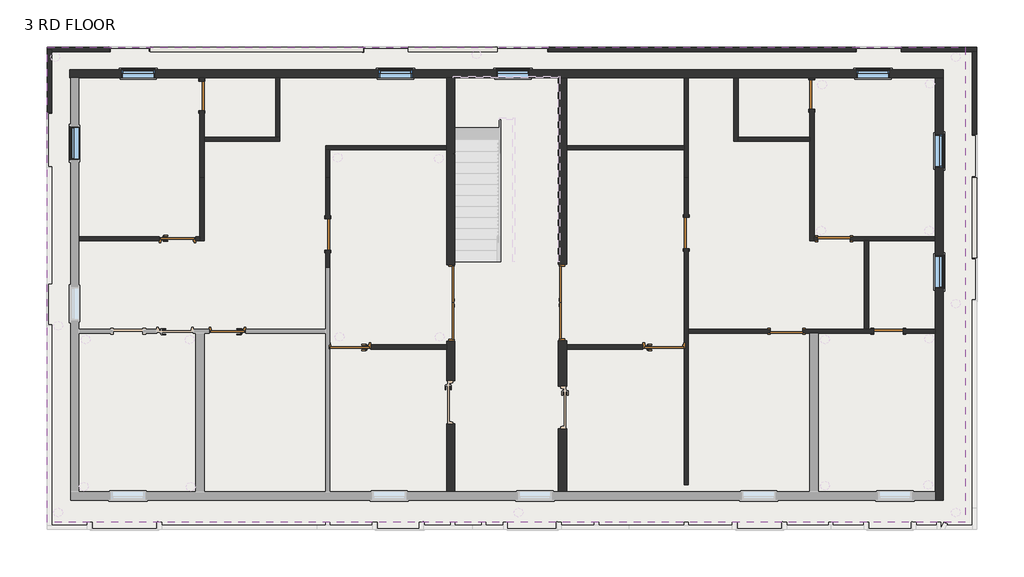
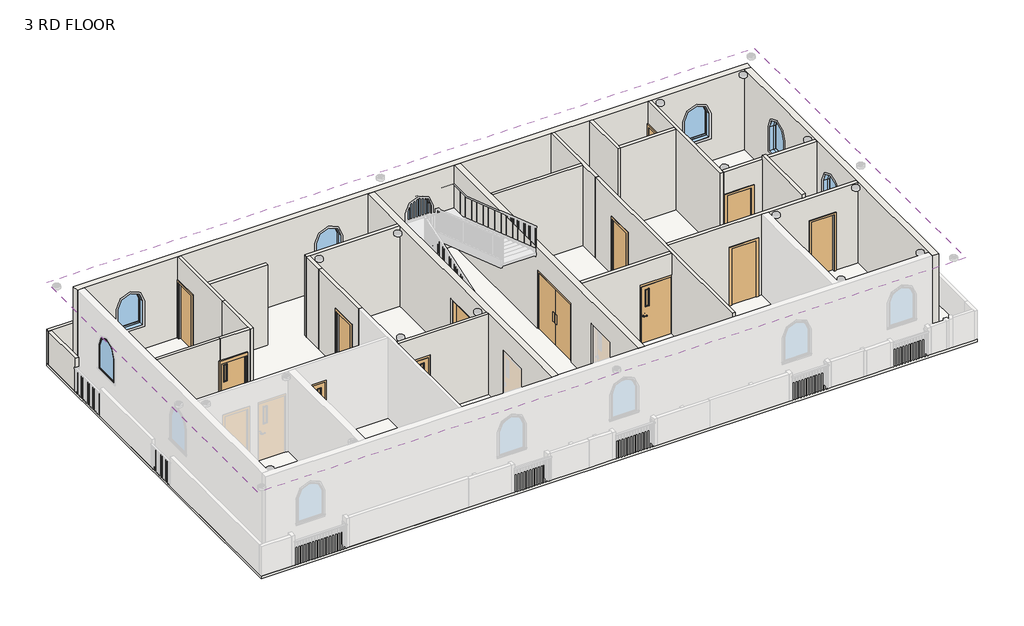
# One storey, part 2 of 7: 33 walls, 13 doors, 7 windows, 1 covering, 1 slab.
# Revit data of these elements (continued)
# Elements 4, 5 (IfcDoor, "Door-Passage-Single-Vision_Lite : 3'6\"X7' 2")
#   Swing Angle = 90.00°
#   Rough Width = 3' - 10"
#   Rough Height = 7' - 4"
#   Masonry Inset = 0' - 1"
#   MFOpeningWidth = 0' - 4"
#   MFOpeningHeight = 0' - 4"
#   Inset Calculate = 0' - 4"
#   Masonry Frame = yes
#   Dry Wall Frame = no
#   Phase Created = New Construction
#   Materials on its faces: "Metal - Paint Finish - Grey", "Aluminum", "Wood - Birch", "Glass"
# Elements 6, 7 (IfcDoor, "Door-Passage-Single-Vision_Lite : 3'X7'")
#   Swing Angle = 90.00°
#   Rough Width = 3' - 4"
#   Rough Height = 7' - 4"
#   Masonry Inset = 0' - 1"
#   MFOpeningWidth = 0' - 4"
#   MFOpeningHeight = 0' - 4"
#   Inset Calculate = 0' - 4"
#   Masonry Frame = yes
#   Dry Wall Frame = no
#   Phase Created = New Construction
#   Materials on its faces: "Metal - Paint Finish - Grey", "Aluminum", "Wood - Birch", "Glass"
# Elements 8, 9 (IfcDoor, "Single-Flush : 2'10\" x 7'")
#   Phase Created = New Construction
#   Materials on its faces: "Door - Frame", "Door - Panel"
# Elements 10, 11 (IfcDoor, "Single-Flush : 2'11\"x 7'")
#   Phase Created = New Construction
#   Materials on its faces: "Door - Frame", "Door - Panel"
# Elements 12, 13, 14 (IfcDoor, "Single-Flush : 2'8\"x 7'")
#   Phase Created = New Construction
#   Materials on its faces: "Door - Frame", "Door - Panel"
# Element 15 (IfcSlab, "LW Concrete on Metal Deck")
#   Height Offset From Level = 0' - 0"
#   Phase Created = New Construction
#   Materials on its faces: "Metal Deck", "Concrete, Lightweight"
# Elements 16, 17, 18, 19, 20, 21, 22, 23, 24, 25, 26, 27, 28, 29, 30, 32, 33, 34 (IfcWall, "Generic - 4.5\"")
#   Top Offset = -0' - 6"
#   Base Offset = 0' - 0"
#   wall height = 10' - 0"
#   Phase Created = New Construction
#   Base Constraint = 3 RD FLOOR
#   Top Constraint = 4 TH FLOOR
#   Materials on its faces: "Default Wall"
# Elements 31, 41 (IfcWall, "Generic - 4.5\"")
#   Top Offset = -6' - 0"
#   Base Offset = 0' - 0"
#   wall height = 4' - 6"
#   Phase Created = New Construction
#   Base Constraint = 3 RD FLOOR
#   Top Constraint = 4 TH FLOOR
#   Materials on its faces: "Default Wall"
# Element 35 (IfcWall, "Generic - 4.5\"")
#   Top Offset = -6' - 4.43284"
#   Base Offset = 0' - 0"
#   wall height = 4' - 1.56716"
#   Phase Created = New Construction
#   Base Constraint = 3 RD FLOOR
#   Top Constraint = 4 TH FLOOR
#   Materials on its faces: "Default Wall"
# Element 36 (IfcWall, "Generic - 4.5\"")
#   Top Offset = -6' - 3.86561"
#   Base Offset = 0' - 0"
#   wall height = 4' - 2.13439"
#   Phase Created = New Construction
#   Base Constraint = 3 RD FLOOR
#   Top Constraint = 4 TH FLOOR
#   Materials on its faces: "Default Wall"
# Element 37 (IfcWall, "Generic - 4.5\"")
#   Top Offset = -6' - 11.32684"
#   Base Offset = 0' - 0"
#   wall height = 3' - 6.67316"
#   Phase Created = New Construction
#   Base Constraint = 3 RD FLOOR
#   Top Constraint = 4 TH FLOOR
#   Materials on its faces: "Default Wall"
# Element 38 (IfcWall, "Generic - 4.5\"")
#   Top Offset = -6' - 6.91444"
#   Base Offset = 0' - 0"
#   wall height = 3' - 11.08556"
#   Phase Created = New Construction
#   Base Constraint = 3 RD FLOOR
#   Top Constraint = 4 TH FLOOR
#   Materials on its faces: "Default Wall"
# Element 39 (IfcWall, "Generic - 4.5\"")
#   Top Offset = -6' - 3.83516"
#   Base Offset = 0' - 0"
#   wall height = 4' - 2.16484"
#   Phase Created = New Construction
#   Base Constraint = 3 RD FLOOR
#   Top Constraint = 4 TH FLOOR
#   Materials on its faces: "Default Wall"
# Element 40 (IfcWall, "Generic - 4.5\"")
#   Top Offset = -6' - 0.2303"
#   Base Offset = 0' - 0"
#   wall height = 4' - 5.7697"
#   Phase Created = New Construction
#   Base Constraint = 3 RD FLOOR
#   Top Constraint = 4 TH FLOOR
#   Materials on its faces: "Default Wall"
# Element 42 (IfcWall, "Generic - 4.5\"")
#   Top Offset = -6' - 7.02989"
#   Base Offset = 0' - 0"
#   wall height = 3' - 10.97011"
#   Phase Created = New Construction
#   Base Constraint = 3 RD FLOOR
#   Top Constraint = 4 TH FLOOR
#   Materials on its faces: "Default Wall"
# Elements 43, 44, 45, 46 (IfcWall, "Generic - 9\"")
#   Top Offset = -0' - 6"
#   Base Offset = 0' - 0"
#   wall height = 10' - 0"
#   Phase Created = New Construction
#   Base Constraint = 3 RD FLOOR
#   Top Constraint = 4 TH FLOOR
#   Materials on its faces: "Concrete Masonry Units"
# Elements 47, 48 (IfcWall, "Interior - 5\" Partition (2-hr)")
#   Top Offset = 0' - 0"
#   Base Offset = 0' - 0"
#   wall height = 10' - 6"
#   Phase Created = New Construction
#   Base Constraint = 3 RD FLOOR
#   Top Constraint = 4 TH FLOOR
#   Materials on its faces: "Default Wall", "Gypsum Wall Board"
# Element 49 (IfcWindow, "Window-Fixed-Round-Top : 3' x 4'")
#   Mark = "150"
#   Window Inset = 0' - 0"
#   Interior Wall Closure = 0' - 2 1/4"
#   Frame Extension = 0' - 0 1/4"
#   Exterior Wall Closure = 0' - 1 1/4"
#   Interior Trim Visibility = yes
#   Exterior Trim Visibility = yes
#   Phase Created = New Construction
#   Materials on its faces: "Wood - Stained", "Clad - White", "Glass"
# Element 50 (IfcWindow, "Window-Fixed-Round-Top : 3' x 4'")
#   Mark = "151"
#   Window Inset = 0' - 0"
#   Interior Wall Closure = 0' - 2 1/4"
#   Frame Extension = 0' - 0 1/4"
#   Exterior Wall Closure = 0' - 1 1/4"
#   Interior Trim Visibility = yes
#   Exterior Trim Visibility = yes
#   Phase Created = New Construction
#   Materials on its faces: "Wood - Stained", "Clad - White", "Glass"
# Element 51 (IfcWindow, "Window-Fixed-Round-Top : 3' x 4'")
#   Mark = "152"
#   Window Inset = 0' - 0"
#   Interior Wall Closure = 0' - 2 1/4"
#   Frame Extension = 0' - 0 1/4"
#   Exterior Wall Closure = 0' - 1 1/4"
#   Interior Trim Visibility = yes
#   Exterior Trim Visibility = yes
#   Phase Created = New Construction
#   Materials on its faces: "Wood - Stained", "Clad - White", "Glass"
# Element 52 (IfcWindow, "Window-Fixed-Round-Top : 3' x 4'")
#   Mark = "153"
#   Window Inset = 0' - 0"
#   Interior Wall Closure = 0' - 2 1/4"
#   Frame Extension = 0' - 0 1/4"
#   Exterior Wall Closure = 0' - 1 1/4"
#   Interior Trim Visibility = yes
#   Exterior Trim Visibility = yes
#   Phase Created = New Construction
#   Materials on its faces: "Wood - Stained", "Clad - White", "Glass"
# Element 53 (IfcWindow, "Window-Fixed-Round-Top : 3' x 4'")
#   Mark = "154"
#   Window Inset = 0' - 0"
#   Interior Wall Closure = 0' - 2 1/4"
#   Frame Extension = 0' - 0 1/4"
#   Exterior Wall Closure = 0' - 1 1/4"
#   Interior Trim Visibility = yes
#   Exterior Trim Visibility = yes
#   Phase Created = New Construction
#   Materials on its faces: "Wood - Stained", "Clad - White", "Glass"
# Element 54 (IfcWindow, "Window-Fixed-Round-Top : 3' x 4'")
#   Mark = "155"
#   Window Inset = 0' - 0"
#   Interior Wall Closure = 0' - 2 1/4"
#   Frame Extension = 0' - 0 1/4"
#   Exterior Wall Closure = 0' - 1 1/4"
#   Interior Trim Visibility = yes
#   Exterior Trim Visibility = yes
#   Phase Created = New Construction
#   Materials on its faces: "Wood - Stained", "Clad - White", "Glass"
# Element 55 (IfcWindow, "Window-Fixed-Round-Top : 3' x 4'")
#   Mark = "156"
#   Window Inset = 0' - 0"
#   Interior Wall Closure = 0' - 2 1/4"
#   Frame Extension = 0' - 0 1/4"
#   Exterior Wall Closure = 0' - 1 1/4"
#   Interior Trim Visibility = yes
#   Exterior Trim Visibility = yes
#   Phase Created = New Construction
#   Materials on its faces: "Wood - Stained", "Clad - White", "Glass"
# Materials
#   "Default": colour RGB 127 127 127, transparency 0, Cost = 0
#   "Acoustic Ceiling Tile 24 x 48": class "Generic", colour RGB 229 229 229, transparency 0, Description = "Acoustic Ceiling Tile 24 x 48", Cost = 0
#   "Metal - Paint Finish - Brindle": class "Paint", colour RGB 164 133 98, transparency 0, Cost = 0
#   "Metal - Paint Finish - Grey": class "Paint", colour RGB 104 104 104, transparency 0, Cost = 0
#   "Aluminium": class "Metal", colour RGB 244 244 244, transparency 0, Description = "Aluminum 6061", Cost = 0
#   "Wood - Birch": class "Wood", colour RGB 166 116 52, transparency 0, Cost = 0
#   "Glass": class "Glass", colour RGB 0 128 192, transparency 0.75, Description = "Soda Lime Glass", Cost = 0
#   "Aluminum": class "Metal", colour RGB 247 247 247, transparency 0, Description = "Aluminum 6061", Cost = 0
#   "Door - Panel": class "Wood", colour RGB 210 159 95, transparency 0, Cost = 0
#   "Door - Frame": colour RGB 118 70 51, transparency 0, Cost = 0
#   "Concrete, Lightweight": class "Concrete", colour RGB 142 141 140, transparency 0, Description = "Lightweight concrete", Cost = 0
#   "Metal Deck": class "Metal", colour RGB 199 199 199, transparency 0, Description = "Steel, mill finish", Cost = 0
#   "Concrete Masonry Units": class "Masonry", colour RGB 227 227 227, transparency 0, Description = "Concrete masonry units", Cost = 0
#   "Gypsum Wall Board": class "Generic", colour RGB 127 127 127, transparency 0, Description = "Gypsum Wall Board", Cost = 0
#   "Metal Stud Layer": class "Metal", colour RGB 199 199 199, transparency 0, Description = "Light gauge steel framing, thermal air layer", Cost = 0
#   "Wood - Stained": class "Wood", colour RGB 224 178 126, transparency 0, Cost = 0
#   "Clad - White": class "Wood", colour RGB 242 242 238, transparency 0, Cost = 0
#   "Default Wall": colour RGB 128 128 128, transparency 0, Cost = 0
